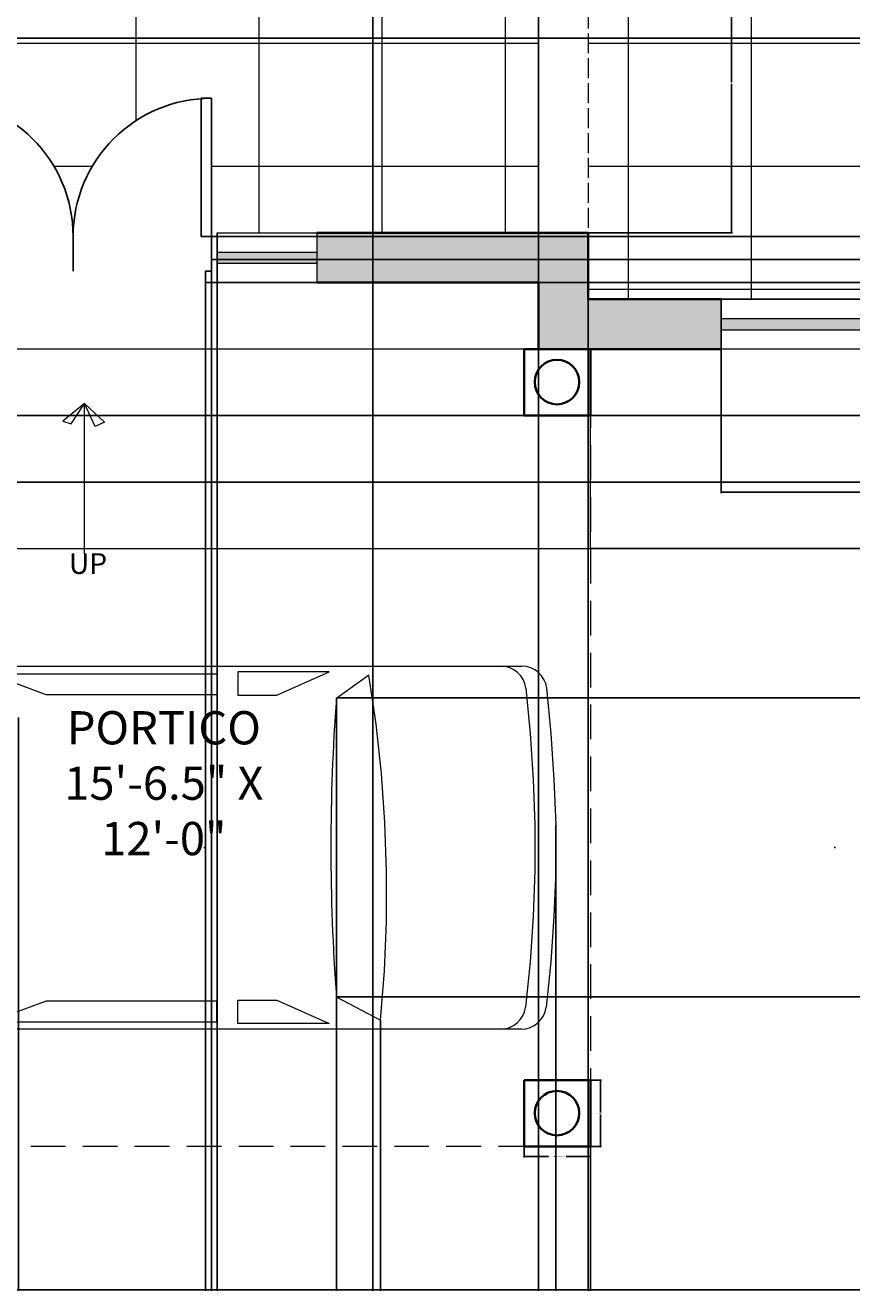
# Model space of a CAD drawing. Units: inches. Extents: x 6 to 575, y 34 to 566.
# Tile 13 of 21: x 282 to 431, y 34 to 262. Entities that reach past the tile are written whole.
import ezdxf

# ---------------------------------------------------------------- set-up
doc = ezdxf.new("R2010")
doc.units = ezdxf.units.IN
doc.linetypes.add('ACAD_ISO02W100', pattern=[15, 12, -3])
for name, color, linetype, lineweight in [('A-ANNO-DIMS', 2, 'Continuous', 18), ('A-ANNO-SYMB', 6, 'Continuous', 18), ('A-ANNO-TEXT', 6, 'Continuous', 18), ('A-AREA-IDEN', 6, 'Continuous', 20), ('A-COLS', 7, 'Continuous', 35), ('A-FLOR-PATT', 252, 'Continuous', 9), ('A-GLAZ-PATT', 4, 'Continuous', 9), ('A-ROOF-OVHD', 240, 'ACAD_ISO02W100', 13), ('A-WALL-OVHD', 7, 'ACAD_ISO02W100', 18), ('A-WALL-PATT', 251, 'Continuous', 9), ('CARS', 5, 'Continuous', 18), ('DOORS', 3, 'Continuous', 25), ('STAIRS', 1, 'Continuous', 20), ('WALLS', 7, 'Continuous', 35), ('WINDOWS', 4, 'Continuous', 20)]:
    doc.layers.add(name, color=color, linetype=linetype, lineweight=lineweight)
doc.styles.add('PDF Arial Narrow', font='txt')
doc.styles.add('PDF Century Gothic', font='txt')
doc.styles.get("Standard").update_dxf_attribs({"font": 'arial.ttf'})
doc.dimstyles.get("Standard").update_dxf_attribs({"dimtxt": 0.18, "dimasz": 0.18, "dimexe": 0.18, "dimexo": 0.0625, "dimgap": 0.09, "dimtad": 0, "dimtih": 1, "dimtoh": 1, "dimdec": 4, "dimzin": 0, "dimdsep": 46, "dimtxsty": 'Standard', "dimcen": 0.09, "dimadec": 0, "dimazin": 0, "dimtfac": 1, "dimtdec": 4, "dimtofl": 0, "dimtmove": 0, "dimatfit": 3, "dimfxl": 1, "dimtolj": 1, "dimtzin": 0, "dimarcsym": 0})
pattern_1 = [(0, (-98.035, 170.147), (0, 22.225), []), (90, (-98.035, 170.147), (-22.225, 1e-15), [])]

# ---------------------------------------------------------------- blocks, each defined once
blk = doc.blocks.new('*U4')
for p, q in [((0, 0), (0, -6)), ((24, 0), (24, -6))]:
    blk.add_line(p, q)
blk.add_lwpolyline([(0, 0), (0, 24), (1.75, 24), (1.75, 0)], close=True)
blk.add_arc((0, 0), 24, 0, 90)
blk = doc.blocks.new('WIN-SIDELIGHT-18IN')
for p, q in [((0, 9), (0, 0)), ((0, 0), (0, 9)), ((0, 9), (0, 0)), ((18, 9), (18, 0)), ((0, 5.5), (18, 5.5)), ((0, 3.5), (18, 3.5))]:
    blk.add_line(p, q)
blk.add_lwpolyline([(0, 9), (18, 9), (18, 0), (0, 0)], close=True)
blk = doc.blocks.new('COL-PORTICO-SQUARE-BASE')
blk.add_lwpolyline([(0, 12.01), (12.02, 12.01), (12.02, 0), (0, 0)], close=True)
blk.add_circle((5.95, 6.05), 4.02)
blk = doc.blocks.new('*D25')
at = {"layer": 'A-ANNO-DIMS', "color": 0, "lineweight": -2, "transparency": 16777216}
for p, q in [((372.06, 59.71), (372.06, 57.79)), ((384.08, 59.71), (384.08, 57.79)), ((372.24, 57.97), (376.47, 57.97)), ((383.9, 57.97), (379.67, 57.97))]:
    blk.add_line(p, q, dxfattribs=at)
at = {"layer": 'A-ANNO-DIMS', "color": 0, "transparency": 16777216}
for points in [[(372.24, 58), (372.24, 57.94), (372.06, 57.97)], [(383.9, 58), (383.9, 57.94), (384.08, 57.97)]]:
    blk.add_solid(points, dxfattribs=at)
at = {"layer": 'Defpoints', "color": 0, "transparency": 16777216}
for p in [(372.06, 59.77), (384.08, 59.78), (384.08, 57.97)]:
    blk.add_point(p, dxfattribs=at)
at = {"layer": 'A-ANNO-DIMS', "color": 0, "transparency": 16777216, "insert": (378.07, 57.97), "char_height": 0.18, "attachment_point": 5}
blk.add_mtext('\\A1;COLUMN BASE R 12 TYP.', dxfattribs=at)
blk = doc.blocks.new('*D26')
at = {"layer": 'A-ANNO-DIMS', "color": 0, "lineweight": -2, "transparency": 16777216}
for p, q in [((384.14, 71.79), (386.06, 71.79)), ((385.88, 71.61), (385.88, 65.96)), ((385.88, 59.96), (385.88, 65.6)), ((384.14, 59.78), (386.06, 59.78))]:
    blk.add_line(p, q, dxfattribs=at)
at = {"layer": 'A-ANNO-DIMS', "color": 0, "transparency": 16777216}
for points in [[(385.91, 71.61), (385.85, 71.61), (385.88, 71.79)], [(385.91, 59.96), (385.85, 59.96), (385.88, 59.78)]]:
    blk.add_solid(points, dxfattribs=at)
at = {"layer": 'Defpoints', "color": 0, "transparency": 16777216}
for p in [(384.07, 71.79), (385.88, 71.79), (384.08, 59.78)]:
    blk.add_point(p, dxfattribs=at)
at = {"layer": 'A-ANNO-DIMS', "color": 0, "transparency": 16777216, "insert": (385.88, 65.78), "char_height": 0.18, "attachment_point": 5}
blk.add_mtext('\\A1;12 TYP.', dxfattribs=at)
blk = doc.blocks.new('*D29')
at = {"layer": 'A-ANNO-DIMS', "color": 0, "lineweight": -2, "transparency": 16777216}
for p, q in [((32.66, 203.74), (32.66, 33.76)), ((548.66, 203.74), (548.66, 33.76)), ((32.84, 33.94), (290.37, 33.94)), ((548.48, 33.94), (290.95, 33.94))]:
    blk.add_line(p, q, dxfattribs=at)
at = {"layer": 'A-ANNO-DIMS', "color": 0, "transparency": 16777216}
for points in [[(32.84, 33.97), (32.84, 33.91), (32.66, 33.94)], [(548.48, 33.97), (548.48, 33.91), (548.66, 33.94)]]:
    blk.add_solid(points, dxfattribs=at)
at = {"layer": 'Defpoints', "color": 0, "transparency": 16777216}
for p in [(32.66, 203.8), (548.66, 203.8), (548.66, 33.94)]:
    blk.add_point(p, dxfattribs=at)
at = {"layer": 'A-ANNO-DIMS', "color": 0, "transparency": 16777216, "insert": (290.66, 33.94), "char_height": 0.18, "attachment_point": 5}
blk.add_mtext('\\A1;516', dxfattribs=at)
blk = doc.blocks.new('*D40')
at = {"layer": 'A-ANNO-DIMS', "color": 0, "lineweight": -2, "transparency": 16777216}
for p, q in [((407.66, 203.74), (407.66, 177.79)), ((515.66, 203.74), (515.66, 177.79)), ((407.84, 177.97), (461.38, 177.97)), ((515.48, 177.97), (461.94, 177.97))]:
    blk.add_line(p, q, dxfattribs=at)
at = {"layer": 'A-ANNO-DIMS', "color": 0, "transparency": 16777216}
for points in [[(407.84, 178), (407.84, 177.94), (407.66, 177.97)], [(515.48, 178), (515.48, 177.94), (515.66, 177.97)]]:
    blk.add_solid(points, dxfattribs=at)
at = {"layer": 'Defpoints', "color": 0, "transparency": 16777216}
for p in [(407.66, 203.8), (515.66, 203.8), (407.66, 177.97)]:
    blk.add_point(p, dxfattribs=at)
at = {"layer": 'A-ANNO-DIMS', "color": 0, "transparency": 16777216, "insert": (461.66, 177.97), "char_height": 0.18, "attachment_point": 5}
blk.add_mtext('\\A1;108', dxfattribs=at)
blk = doc.blocks.new('*D48')
at = {"layer": 'A-ANNO-DIMS', "color": 0, "lineweight": -2, "transparency": 16777216}
for p, q in [((264.66, 215.74), (264.66, 33.76)), ((316.66, 215.74), (316.66, 33.76)), ((264.84, 33.94), (290.44, 33.94)), ((316.48, 33.94), (290.88, 33.94))]:
    blk.add_line(p, q, dxfattribs=at)
at = {"layer": 'A-ANNO-DIMS', "color": 0, "transparency": 16777216}
for points in [[(264.84, 33.97), (264.84, 33.91), (264.66, 33.94)], [(316.48, 33.97), (316.48, 33.91), (316.66, 33.94)]]:
    blk.add_solid(points, dxfattribs=at)
at = {"layer": 'Defpoints', "color": 0, "transparency": 16777216}
for p in [(264.66, 215.8), (316.66, 215.8), (316.66, 33.94)]:
    blk.add_point(p, dxfattribs=at)
at = {"layer": 'A-ANNO-DIMS', "color": 0, "transparency": 16777216, "insert": (290.66, 33.94), "char_height": 0.18, "attachment_point": 5}
blk.add_mtext('\\A1;52', dxfattribs=at)
blk = doc.blocks.new('*D54')
at = {"layer": 'A-ANNO-DIMS', "color": 0, "lineweight": -2, "transparency": 16777216}
for p, q in [((444.96, 337.94), (6.65, 337.94)), ((6.83, 337.76), (6.83, 299.11)), ((6.83, 260.1), (6.83, 298.75)), ((444.96, 259.92), (6.65, 259.92))]:
    blk.add_line(p, q, dxfattribs=at)
at = {"layer": 'A-ANNO-DIMS', "color": 0, "transparency": 16777216}
for points in [[(6.8, 337.76), (6.86, 337.76), (6.83, 337.94)], [(6.8, 260.1), (6.86, 260.1), (6.83, 259.92)]]:
    blk.add_solid(points, dxfattribs=at)
at = {"layer": 'Defpoints', "color": 0, "transparency": 16777216}
for p in [(6.83, 337.94), (445.02, 337.94), (445.02, 259.92)]:
    blk.add_point(p, dxfattribs=at)
at = {"layer": 'A-ANNO-DIMS', "color": 0, "transparency": 16777216, "insert": (6.83, 298.93), "char_height": 0.18, "attachment_point": 5}
blk.add_mtext('\\A1;78.02', dxfattribs=at)
blk = doc.blocks.new('*D58')
at = {"layer": 'A-ANNO-DIMS', "color": 0, "lineweight": -2, "transparency": 16777216}
for p, q in [((383.72, 278.8), (409.67, 278.8)), ((409.49, 278.62), (409.49, 251.98)), ((409.49, 224.98), (409.49, 251.62)), ((383.72, 224.8), (409.67, 224.8))]:
    blk.add_line(p, q, dxfattribs=at)
at = {"layer": 'A-ANNO-DIMS', "color": 0, "transparency": 16777216}
for points in [[(409.46, 278.62), (409.52, 278.62), (409.49, 278.8)], [(409.46, 224.98), (409.52, 224.98), (409.49, 224.8)]]:
    blk.add_solid(points, dxfattribs=at)
at = {"layer": 'Defpoints', "color": 0, "transparency": 16777216}
for p in [(383.66, 278.8), (383.66, 224.8), (409.49, 224.8)]:
    blk.add_point(p, dxfattribs=at)
at = {"layer": 'A-ANNO-DIMS', "color": 0, "transparency": 16777216, "insert": (409.49, 251.8), "char_height": 0.18, "attachment_point": 5}
blk.add_mtext('\\A1;54', dxfattribs=at)
blk = doc.blocks.new('*D74')
at = {"layer": 'A-ANNO-DIMS', "color": 0, "lineweight": -2, "transparency": 16777216}
for p, q in [((384.14, 191.79), (574.68, 191.79)), ((574.5, 191.61), (574.5, 185.96)), ((574.5, 179.95), (574.5, 185.6)), ((384.14, 179.77), (574.68, 179.77))]:
    blk.add_line(p, q, dxfattribs=at)
at = {"layer": 'A-ANNO-DIMS', "color": 0, "transparency": 16777216}
for points in [[(574.47, 191.61), (574.53, 191.61), (574.5, 191.79)], [(574.47, 179.95), (574.53, 179.95), (574.5, 179.77)]]:
    blk.add_solid(points, dxfattribs=at)
at = {"layer": 'Defpoints', "color": 0, "transparency": 16777216}
for p in [(384.08, 191.79), (384.08, 179.77), (574.5, 179.77)]:
    blk.add_point(p, dxfattribs=at)
at = {"layer": 'A-ANNO-DIMS', "color": 0, "transparency": 16777216, "insert": (574.5, 185.78), "char_height": 0.18, "attachment_point": 5}
blk.add_mtext('\\A1;12.015', dxfattribs=at)
blk = doc.blocks.new('*D75')
at = {"layer": 'A-ANNO-DIMS', "color": 0, "lineweight": -2, "transparency": 16777216}
for p, q in [((384.14, 179.77), (574.68, 179.77)), ((574.5, 179.59), (574.5, 173.95)), ((574.5, 167.94), (574.5, 173.58)), ((384.14, 167.76), (574.68, 167.76))]:
    blk.add_line(p, q, dxfattribs=at)
at = {"layer": 'A-ANNO-DIMS', "color": 0, "transparency": 16777216}
for points in [[(574.47, 179.59), (574.53, 179.59), (574.5, 179.77)], [(574.47, 167.94), (574.53, 167.94), (574.5, 167.76)]]:
    blk.add_solid(points, dxfattribs=at)
at = {"layer": 'Defpoints', "color": 0, "transparency": 16777216}
for p in [(384.08, 179.77), (384.08, 167.76), (574.5, 167.76)]:
    blk.add_point(p, dxfattribs=at)
at = {"layer": 'A-ANNO-DIMS', "color": 0, "transparency": 16777216, "insert": (574.5, 173.76), "char_height": 0.18, "attachment_point": 5}
blk.add_mtext('\\A1;12.015', dxfattribs=at)
blk = doc.blocks.new('*D76')
at = {"layer": 'A-ANNO-DIMS', "color": 0, "lineweight": -2, "transparency": 16777216}
for p, q in [((197.69, 59.71), (197.69, 33.76)), ((384.08, 59.71), (384.08, 33.76)), ((197.87, 33.94), (290.5, 33.94)), ((383.9, 33.94), (291.27, 33.94))]:
    blk.add_line(p, q, dxfattribs=at)
at = {"layer": 'A-ANNO-DIMS', "color": 0, "transparency": 16777216}
for points in [[(197.87, 33.97), (197.87, 33.91), (197.69, 33.94)], [(383.9, 33.97), (383.9, 33.91), (384.08, 33.94)]]:
    blk.add_solid(points, dxfattribs=at)
at = {"layer": 'Defpoints', "color": 0, "transparency": 16777216}
for p in [(197.69, 59.77), (384.08, 59.78), (384.08, 33.94)]:
    blk.add_point(p, dxfattribs=at)
at = {"layer": 'A-ANNO-DIMS', "color": 0, "transparency": 16777216, "insert": (290.88, 33.94), "char_height": 0.18, "attachment_point": 5}
blk.add_mtext('\\A1;186.4', dxfattribs=at)
blk = doc.blocks.new('*D78')
at = {"layer": 'A-ANNO-DIMS', "color": 0, "lineweight": -2, "transparency": 16777216}
for p, q in [((377.83, 117.84), (377.83, 33.76)), ((206.58, 113.74), (206.58, 33.76)), ((206.76, 33.94), (291.75, 33.94)), ((377.65, 33.94), (292.66, 33.94))]:
    blk.add_line(p, q, dxfattribs=at)
at = {"layer": 'A-ANNO-DIMS', "color": 0, "transparency": 16777216}
for points in [[(206.76, 33.97), (206.76, 33.91), (206.58, 33.94)], [(377.65, 33.97), (377.65, 33.91), (377.83, 33.94)]]:
    blk.add_solid(points, dxfattribs=at)
at = {"layer": 'Defpoints', "color": 0, "transparency": 16777216}
for p in [(377.83, 117.9), (206.58, 113.81), (377.83, 33.94)]:
    blk.add_point(p, dxfattribs=at)
at = {"layer": 'A-ANNO-DIMS', "color": 0, "transparency": 16777216, "insert": (292.21, 33.94), "char_height": 0.18, "attachment_point": 5}
blk.add_mtext('\\A1;171.25', dxfattribs=at)
blk = doc.blocks.new('*D82')
at = {"layer": 'A-ANNO-DIMS', "color": 0, "lineweight": -2, "transparency": 16777216}
for p, q in [((338.25, 140.81), (574.68, 140.81)), ((574.5, 140.63), (574.5, 113.99)), ((574.5, 86.98), (574.5, 113.62)), ((338.25, 86.8), (574.68, 86.8))]:
    blk.add_line(p, q, dxfattribs=at)
at = {"layer": 'A-ANNO-DIMS', "color": 0, "transparency": 16777216}
for points in [[(574.47, 140.63), (574.53, 140.63), (574.5, 140.81)], [(574.47, 86.98), (574.53, 86.98), (574.5, 86.8)]]:
    blk.add_solid(points, dxfattribs=at)
at = {"layer": 'Defpoints', "color": 0, "transparency": 16777216}
for p in [(338.19, 140.81), (574.5, 140.81), (338.19, 86.8)]:
    blk.add_point(p, dxfattribs=at)
at = {"layer": 'A-ANNO-DIMS', "color": 0, "transparency": 16777216, "insert": (574.5, 113.81), "char_height": 0.18, "attachment_point": 5}
blk.add_mtext('\\A1;54.02', dxfattribs=at)
blk = doc.blocks.new('*D85')
at = {"layer": 'A-ANNO-DIMS', "color": 0, "lineweight": -2, "transparency": 16777216}
for p, q in [((338.19, 140.75), (338.19, 33.76)), ((280.78, 137.27), (280.78, 33.76)), ((280.96, 33.94), (309.11, 33.94)), ((338.01, 33.94), (309.86, 33.94))]:
    blk.add_line(p, q, dxfattribs=at)
at = {"layer": 'A-ANNO-DIMS', "color": 0, "transparency": 16777216}
for points in [[(280.96, 33.97), (280.96, 33.91), (280.78, 33.94)], [(338.01, 33.97), (338.01, 33.91), (338.19, 33.94)]]:
    blk.add_solid(points, dxfattribs=at)
at = {"layer": 'Defpoints', "color": 0, "transparency": 16777216}
for p in [(338.19, 140.81), (280.78, 137.33), (338.19, 33.94)]:
    blk.add_point(p, dxfattribs=at)
at = {"layer": 'A-ANNO-DIMS', "color": 0, "transparency": 16777216, "insert": (309.48, 33.94), "char_height": 0.18, "attachment_point": 5}
blk.add_mtext('\\A1;57.41', dxfattribs=at)
blk = doc.blocks.new('*D86')
at = {"layer": 'A-ANNO-DIMS', "color": 0, "lineweight": -2, "transparency": 16777216}
for p, q in [((338.19, 86.73), (338.19, 33.76)), ((346.16, 82.57), (346.16, 33.76)), ((338.37, 33.94), (341.78, 33.94)), ((345.98, 33.94), (342.57, 33.94))]:
    blk.add_line(p, q, dxfattribs=at)
at = {"layer": 'A-ANNO-DIMS', "color": 0, "transparency": 16777216}
for points in [[(338.37, 33.97), (338.37, 33.91), (338.19, 33.94)], [(345.98, 33.97), (345.98, 33.91), (346.16, 33.94)]]:
    blk.add_solid(points, dxfattribs=at)
at = {"layer": 'Defpoints', "color": 0, "transparency": 16777216}
for p in [(338.19, 86.8), (346.16, 82.64), (346.16, 33.94)]:
    blk.add_point(p, dxfattribs=at)
at = {"layer": 'A-ANNO-DIMS', "color": 0, "transparency": 16777216, "insert": (342.17, 33.94), "char_height": 0.18, "attachment_point": 5}
blk.add_mtext('\\A1;7.967', dxfattribs=at)
blk = doc.blocks.new('*D122')
at = {"layer": 'A-ANNO-DIMS', "color": 0, "lineweight": -2, "transparency": 16777216}
for p, q in [((344.78, 281.17), (344.78, 33.76)), ((374.66, 278.74), (374.66, 33.76)), ((344.96, 33.94), (359.32, 33.94)), ((374.48, 33.94), (360.11, 33.94))]:
    blk.add_line(p, q, dxfattribs=at)
at = {"layer": 'A-ANNO-DIMS', "color": 0, "transparency": 16777216}
for points in [[(344.96, 33.97), (344.96, 33.91), (344.78, 33.94)], [(374.48, 33.97), (374.48, 33.91), (374.66, 33.94)]]:
    blk.add_solid(points, dxfattribs=at)
at = {"layer": 'Defpoints', "color": 0, "transparency": 16777216}
for p in [(344.78, 281.24), (374.66, 278.8), (344.78, 33.94)]:
    blk.add_point(p, dxfattribs=at)
at = {"layer": 'A-ANNO-DIMS', "color": 0, "transparency": 16777216, "insert": (359.72, 33.94), "char_height": 0.18, "attachment_point": 5}
blk.add_mtext('\\A1;29.88', dxfattribs=at)
blk = doc.blocks.new('*D138')
at = {"layer": 'A-ANNO-DIMS', "color": 0, "lineweight": -2, "transparency": 16777216}
for p, q in [((445.02, 259.86), (445.02, 33.76)), ((383.66, 212.74), (383.66, 33.76)), ((383.84, 33.94), (413.95, 33.94)), ((444.84, 33.94), (414.73, 33.94))]:
    blk.add_line(p, q, dxfattribs=at)
at = {"layer": 'A-ANNO-DIMS', "color": 0, "transparency": 16777216}
for points in [[(383.84, 33.97), (383.84, 33.91), (383.66, 33.94)], [(444.84, 33.97), (444.84, 33.91), (445.02, 33.94)]]:
    blk.add_solid(points, dxfattribs=at)
at = {"layer": 'Defpoints', "color": 0, "transparency": 16777216}
for p in [(445.02, 259.92), (383.66, 212.8), (445.02, 33.94)]:
    blk.add_point(p, dxfattribs=at)
at = {"layer": 'A-ANNO-DIMS', "color": 0, "transparency": 16777216, "insert": (414.34, 33.94), "char_height": 0.18, "attachment_point": 5}
blk.add_mtext('\\A1;61.36', dxfattribs=at)
blk = doc.blocks.new('*D139')
at = {"layer": 'A-ANNO-DIMS', "color": 0, "lineweight": -2, "transparency": 16777216}
for p, q in [((445.08, 259.92), (574.68, 259.92)), ((574.5, 259.74), (574.5, 236.54)), ((574.5, 212.98), (574.5, 236.18)), ((383.72, 212.8), (574.68, 212.8))]:
    blk.add_line(p, q, dxfattribs=at)
at = {"layer": 'A-ANNO-DIMS', "color": 0, "transparency": 16777216}
for points in [[(574.47, 259.74), (574.53, 259.74), (574.5, 259.92)], [(574.47, 212.98), (574.53, 212.98), (574.5, 212.8)]]:
    blk.add_solid(points, dxfattribs=at)
at = {"layer": 'Defpoints', "color": 0, "transparency": 16777216}
for p in [(445.02, 259.92), (574.5, 259.92), (383.66, 212.8)]:
    blk.add_point(p, dxfattribs=at)
at = {"layer": 'A-ANNO-DIMS', "color": 0, "transparency": 16777216, "insert": (574.5, 236.36), "char_height": 0.18, "attachment_point": 5}
blk.add_mtext('\\A1;47.12', dxfattribs=at)
blk = doc.blocks.new('*D211')
at = {"layer": 'A-ANNO-DIMS', "color": 0, "lineweight": -2, "transparency": 16777216}
for p, q in [((314.58, 215.74), (314.58, 33.76)), ((316.66, 215.74), (316.66, 33.76)), ((314.76, 33.94), (315.29, 33.94)), ((316.48, 33.94), (315.94, 33.94))]:
    blk.add_line(p, q, dxfattribs=at)
at = {"layer": 'A-ANNO-DIMS', "color": 0, "transparency": 16777216}
for points in [[(314.76, 33.97), (314.76, 33.91), (314.58, 33.94)], [(316.48, 33.97), (316.48, 33.91), (316.66, 33.94)]]:
    blk.add_solid(points, dxfattribs=at)
at = {"layer": 'Defpoints', "color": 0, "transparency": 16777216}
for p in [(314.58, 215.8), (316.66, 215.8), (314.58, 33.94)]:
    blk.add_point(p, dxfattribs=at)
at = {"layer": 'A-ANNO-DIMS', "color": 0, "transparency": 16777216, "insert": (315.62, 33.94), "char_height": 0.18, "attachment_point": 5}
blk.add_mtext('\\A1;2.08', dxfattribs=at)
blk = doc.blocks.new('*D212')
at = {"layer": 'A-ANNO-DIMS', "color": 0, "lineweight": -2, "transparency": 16777216}
for p, q in [((316.72, 219.96), (574.68, 219.96)), ((574.5, 219.78), (574.5, 218.06)), ((574.5, 215.98), (574.5, 217.7)), ((316.72, 215.8), (574.68, 215.8))]:
    blk.add_line(p, q, dxfattribs=at)
at = {"layer": 'A-ANNO-DIMS', "color": 0, "transparency": 16777216}
for points in [[(574.47, 219.78), (574.53, 219.78), (574.5, 219.96)], [(574.47, 215.98), (574.53, 215.98), (574.5, 215.8)]]:
    blk.add_solid(points, dxfattribs=at)
at = {"layer": 'Defpoints', "color": 0, "transparency": 16777216}
for p in [(316.66, 219.96), (574.5, 219.96), (316.66, 215.8)]:
    blk.add_point(p, dxfattribs=at)
at = {"layer": 'A-ANNO-DIMS', "color": 0, "transparency": 16777216, "insert": (574.5, 217.88), "char_height": 0.18, "attachment_point": 5}
blk.add_mtext('\\A1;4.16', dxfattribs=at)
blk = doc.blocks.new('*D213')
at = {"layer": 'A-ANNO-DIMS', "color": 0, "lineweight": -2, "transparency": 16777216}
for p, q in [((314.578645, 217.818484), (314.578645, 33.76465)), ((315.618645, 217.818484), (315.618645, 33.76465)), ((314.398645, 33.94465), (314.218645, 33.94465)), ((315.798645, 33.94465), (315.978645, 33.94465))]:
    blk.add_line(p, q, dxfattribs=at)
at = {"layer": 'A-ANNO-DIMS', "color": 0, "transparency": 16777216}
for points in [[(314.398645, 33.97465), (314.398645, 33.91465), (314.578645, 33.94465)], [(315.798645, 33.97465), (315.798645, 33.91465), (315.618645, 33.94465)]]:
    blk.add_solid(points, dxfattribs=at)
at = {"layer": 'Defpoints', "color": 0, "transparency": 16777216}
for p in [(314.578645, 217.880984), (315.618645, 217.880984), (314.578645, 33.94465)]:
    blk.add_point(p, dxfattribs=at)
at = {"layer": 'A-ANNO-DIMS', "color": 0, "transparency": 16777216, "insert": (315.098645, 33.94465), "char_height": 0.18, "attachment_point": 5}
blk.add_mtext('\\A1;1.04', dxfattribs=at)
blk = doc.blocks.new('*D216')
at = {"layer": 'A-ANNO-DIMS', "color": 0, "lineweight": -2, "transparency": 16777216}
for p, q in [((315.68, 224.12), (574.68, 224.12)), ((574.5, 223.94), (574.5, 222.22)), ((574.5, 220.14), (574.5, 221.86)), ((315.68, 219.96), (574.68, 219.96))]:
    blk.add_line(p, q, dxfattribs=at)
at = {"layer": 'A-ANNO-DIMS', "color": 0, "transparency": 16777216}
for points in [[(574.47, 223.94), (574.53, 223.94), (574.5, 224.12)], [(574.47, 220.14), (574.53, 220.14), (574.5, 219.96)]]:
    blk.add_solid(points, dxfattribs=at)
at = {"layer": 'Defpoints', "color": 0, "transparency": 16777216}
for p in [(315.62, 224.12), (574.5, 224.12), (315.62, 219.96)]:
    blk.add_point(p, dxfattribs=at)
at = {"layer": 'A-ANNO-DIMS', "color": 0, "transparency": 16777216, "insert": (574.5, 222.04), "char_height": 0.18, "attachment_point": 5}
blk.add_mtext('\\A1;4.16', dxfattribs=at)
blk = doc.blocks.new('*D220')
at = {"layer": 'A-ANNO-DIMS', "color": 0, "lineweight": -2, "transparency": 16777216}
for p, q in [((155, 113.8), (257.27, 113.8)), ((428.11, 113.81), (428.29, 113.81)), ((428.2, 113.72), (428.2, 113.9))]:
    blk.add_line(p, q, dxfattribs=at)
at = {"layer": 'A-ANNO-DIMS', "color": 0, "transparency": 16777216}
blk.add_solid([(257.27, 113.83), (257.27, 113.77), (257.45, 113.8)], dxfattribs=at)
at = {"layer": 'Defpoints', "color": 0, "transparency": 16777216}
for p in [(257.45, 113.8), (428.2, 113.81)]:
    blk.add_point(p, dxfattribs=at)
at = {"layer": 'A-ANNO-DIMS', "color": 0, "transparency": 16777216, "insert": (154.45, 113.8), "char_height": 0.18, "attachment_point": 5}
blk.add_mtext('\\A1;R170.75', dxfattribs=at)
blk = doc.blocks.new('*D221')
at = {"layer": 'A-ANNO-DIMS', "color": 0, "lineweight": -2, "transparency": 16777216}
for p, q in [((141.91, 113.8), (206.4, 113.8)), ((314.28, 113.81), (314.46, 113.81)), ((314.37, 113.72), (314.37, 113.9))]:
    blk.add_line(p, q, dxfattribs=at)
at = {"layer": 'A-ANNO-DIMS', "color": 0, "transparency": 16777216}
blk.add_solid([(206.4, 113.83), (206.4, 113.77), (206.58, 113.8)], dxfattribs=at)
at = {"layer": 'Defpoints', "color": 0, "transparency": 16777216}
for p in [(206.58, 113.8), (314.37, 113.81)]:
    blk.add_point(p, dxfattribs=at)
at = {"layer": 'A-ANNO-DIMS', "color": 0, "transparency": 16777216, "insert": (141.36, 113.8), "char_height": 0.18, "attachment_point": 5}
blk.add_mtext('\\A1;R107.78', dxfattribs=at)
blk = doc.blocks.new('*D222')
at = {"layer": 'A-ANNO-DIMS', "color": 0, "lineweight": -2, "transparency": 16777216}
for p, q in [((150.38, 113.8), (211.32, 113.8)), ((313.26, 113.81), (313.44, 113.81)), ((313.35, 113.72), (313.35, 113.9))]:
    blk.add_line(p, q, dxfattribs=at)
at = {"layer": 'A-ANNO-DIMS', "color": 0, "transparency": 16777216}
blk.add_solid([(211.32, 113.83), (211.32, 113.77), (211.5, 113.8)], dxfattribs=at)
at = {"layer": 'Defpoints', "color": 0, "transparency": 16777216}
for p in [(211.5, 113.8), (313.35, 113.81)]:
    blk.add_point(p, dxfattribs=at)
at = {"layer": 'A-ANNO-DIMS', "color": 0, "transparency": 16777216, "insert": (149.83, 113.8), "char_height": 0.18, "attachment_point": 5}
blk.add_mtext('\\A1;R101.85', dxfattribs=at)

msp = doc.modelspace()

# ---------------------------------------------------------------- hatches: boundary and pattern name
at = {"layer": 'A-FLOR-PATT'}
h = msp.add_hatch(dxfattribs=at)
h.set_pattern_fill('NET', color=256, scale=7)
h.set_pattern_definition(pattern_1)
h.paths.add_polyline_path([(539.6586, 366.801), (539.6586, 378.801), (433.708, 378.801), (383.6586, 378.801), (383.6586, 278.801), (383.6586, 224.801), (383.6586, 212.801), (407.6586, 212.801), (515.6586, 212.801), (539.6586, 212.801), (539.6586, 270.801)])
h.paths.add_polyline_path([(434.8003, 333.3365), (436.6727, 333.3365), (436.6727, 331.9322), (445.0208, 331.9322), (445.0208, 337.9397), (456.1776, 337.9397), (456.1776, 346.2878), (454.7733, 346.2878), (454.7733, 348.1603), (474.2782, 348.1603), (474.2782, 346.2878), (472.8738, 346.2878), (472.8738, 337.9397), (484.0307, 337.9397), (484.0307, 331.9322), (492.3788, 331.9322), (492.3788, 333.3365), (494.2512, 333.3365), (494.2512, 313.8316), (492.3788, 313.8316), (492.3788, 315.158), (484.0307, 315.158), (484.0307, 307.278), (492.3788, 307.278), (492.3788, 308.6823), (494.2512, 308.6823), (494.2512, 289.1774), (492.3788, 289.1774), (492.3788, 290.5818), (484.0307, 290.5818), (484.0307, 282.7018), (492.3788, 282.7018), (492.3788, 284.1062), (494.2512, 284.1062), (494.2512, 264.6013), (492.3788, 264.6013), (492.3788, 266.0056), (484.0307, 266.0056), (484.0307, 259.9201), (472.8738, 259.9201), (472.8738, 251.572), (474.2782, 251.572), (474.2782, 249.6995), (454.7733, 249.6995), (454.7733, 251.572), (456.1776, 251.572), (456.1776, 259.9201), (445.0208, 259.9201), (445.0208, 266.0056), (436.6727, 266.0056), (436.6727, 264.6013), (434.8003, 264.6013), (434.8003, 284.1062), (436.6727, 284.1062), (436.6727, 282.7018), (445.0208, 282.7018), (445.0208, 290.5818), (436.6727, 290.5818), (436.6727, 289.1774), (434.8003, 289.1774), (434.8003, 308.6823), (436.6727, 308.6823), (436.6727, 307.278), (445.0208, 307.278), (445.0208, 315.158), (436.6727, 315.158), (436.6727, 313.8316), (434.8003, 313.8316)], flags=16)
h.paths.add_polyline_path([(532.9619, 436.5144), (533.9192, 437.0672), (533.9307, 437.0472, -0.12106636), (546.2274, 440.0689), (539.6586, 440.801), (539.6586, 450.6781), (515.7066, 450.6781), (515.7066, 507.3203), (407.6494, 507.3203), (407.6494, 449.3517), (383.6586, 449.3517), (383.6586, 382.801), (433.708, 382.801), (433.708, 406.831), (539.6586, 406.831), (539.6586, 412.801), (545.7108, 412.801), (545.7108, 414.4327)])
h.paths.add_polyline_path([(437.687, 435.3082), (437.687, 471.3533), (485.6691, 471.3533), (485.6691, 435.3082)], flags=16)
h = msp.add_hatch(dxfattribs=at)
h.set_pattern_fill('NET', color=256, scale=7)
h.set_pattern_definition(pattern_1)
h.paths.add_polyline_path([(368.183, 395.6385, -0.88370529), (374.2533, 394.8861), (374.6586, 448.801), (354.6586, 448.801), (354.6586, 448.7938), (353.1847, 448.7938), (326.6586, 448.801), (322.6586, 448.801), (248.6332, 448.8024), (206.6586, 448.8024), (206.6586, 389.449), (221.6622, 389.449), (221.6622, 310.5712), (206.6586, 310.5712), (206.6586, 276.801), (206.6704, 276.801), (206.6704, 274.3795), (206.6586, 224.801), (246.6586, 224.801), (264.6586, 224.801), (265.6986, 224.801), (265.6986, 249.081), (267.5186, 249.081), (267.5186, 249.0145, -0.38515288), (290.6494, 224.801), (290.6679, 224.801, -0.38515288), (313.7986, 249.0145), (313.7986, 249.081), (315.6186, 249.081), (315.6186, 224.801), (316.6586, 224.801), (334.6586, 224.801), (374.6586, 224.801), (374.6586, 278.801), (374.1753, 318.8919, -0.45530286), (370.7577, 315.9168), (370.6643, 313.8205, -0.41421356), (368.7528, 311.909), (368.8072, 311.8975), (368.7528, 311.909, 0.41421356), (370.6643, 313.8205), (370.7632, 315.9161, -0.34634601), (368.183, 318.5897)])
h.paths.add_polyline_path([(288.603, 342.0131), (288.603, 389.9952), (318.6406, 389.9952), (318.6406, 342.0131)], flags=16)
h.paths.add_polyline_path([(289.6173, 343.0274), (289.6173, 389.059), (317.6263, 389.059), (317.6263, 343.0274)], flags=0)
h.paths.add_polyline_path([(295.4867, 311.7535, 0.06538163), (295.1241, 312.0945), (295.0006, 312.1316)], flags=16)
h.paths.add_polyline_path([(328.4931, 284.9911, 0.41421356), (330.4045, 286.9026), (330.4215, 286.8532), (330.4045, 286.9026, -0.41421356), (328.4931, 284.9911), (328.549, 284.9808)], flags=16)
h.paths.add_polyline_path([(344.7771, 305.2659), (368.8072, 305.2659), (368.8072, 281.2358), (344.7771, 281.2358)], flags=16)
h.paths.add_polyline_path([(368.183, 288.1406, -1), (356.246, 288.1406, -1)], flags=0)
h.paths.add_polyline_path([(347.9759, 404.6629), (347.9759, 428.6929), (372.006, 428.6929), (372.006, 404.6629)], flags=16)
h.paths.add_polyline_path([(359.4448, 421.7882, -1), (371.3818, 421.7882, -1)], flags=0)
at = {"layer": 'A-GLAZ-PATT'}
h = msp.add_hatch(color=256, dxfattribs=at)
h.dxf.hatch_style = 1
h.paths.add_polyline_path([(36.1586, 224.801), (38.1586, 224.801), (38.1586, 272.801), (36.1586, 272.801)])
h.paths.add_polyline_path([(167.6586, 207.301), (167.6586, 209.301), (71.6586, 209.301), (71.6586, 207.301)])
h.paths.add_polyline_path([(264.6586, 219.301), (264.6586, 221.301), (246.6586, 221.301), (246.6586, 219.301)])
h.paths.add_polyline_path([(316.6586, 221.301), (316.6586, 219.301), (334.6586, 219.301), (334.6586, 221.301)])
h.paths.add_polyline_path([(515.6586, 207.301), (515.6586, 209.301), (407.6586, 209.301), (407.6586, 207.301)])
h.paths.add_polyline_path([(543.1586, 270.801), (545.1586, 270.801), (545.1586, 366.801), (543.1586, 366.801)])
h.paths.add_polyline_path([(407.9436, 536.301), (407.9436, 534.301), (455.9436, 534.301), (455.9436, 536.301)])
h.paths.add_polyline_path([(272.6586, 536.301), (272.6586, 534.301), (320.6586, 534.301), (320.6586, 536.301)])
at = {"layer": 'A-WALL-PATT'}
h = msp.add_hatch(color=256, dxfattribs=at)
h.dxf.hatch_style = 1
h.paths.add_polyline_path([(160.6586, 539.801), (32.6586, 539.801), (32.6586, 272.801), (41.6586, 272.801), (41.6586, 286.0643), (41.6586, 358.0764), (41.6586, 379.0637), (41.6586, 407.7709), (41.6194, 407.7709), (41.6194, 431.801), (82.8918, 431.801), (82.8918, 440.801), (65.6494, 440.801), (65.6494, 440.7732), (41.6194, 440.7732), (41.6194, 515.5941), (41.6586, 530.801), (117.6586, 530.801), (117.6586, 474.801), (120.6068, 474.801), (121.6586, 474.801), (121.6586, 530.801), (137.4275, 530.801), (137.4275, 530.8356), (141.2505, 530.8356), (160.6586, 530.801)])
h.paths.add_polyline_path([(71.6586, 212.801), (41.6586, 212.801), (41.6586, 224.801), (32.6586, 224.801), (32.6586, 203.801), (71.6586, 203.801)])
h.paths.add_polyline_path([(206.6586, 215.801), (246.6586, 215.801), (246.6586, 224.801), (206.6586, 224.801), (206.6586, 230.801), (201.8157, 230.801), (197.6586, 230.801), (197.6586, 212.801), (167.6586, 212.801), (167.6586, 203.801), (206.6586, 203.801)])
h.paths.add_polyline_path([(383.6586, 224.801), (334.6586, 224.801), (334.6586, 215.801), (374.6586, 215.801), (374.6586, 203.801), (384.0753, 203.801), (407.6586, 203.801), (407.6586, 212.801), (383.6586, 212.801)])
h.paths.add_polyline_path([(548.6586, 270.801), (539.6586, 270.801), (539.6586, 212.801), (515.6586, 212.801), (515.6586, 203.801), (548.6586, 203.801)])
h.paths.add_polyline_path([(548.6586, 412.801), (545.7108, 412.801), (539.6586, 412.801), (539.6586, 382.801), (433.708, 382.801), (433.708, 378.801), (539.6586, 378.801), (539.6586, 366.801), (548.6586, 366.801)])
h.paths.add_polyline_path([(548.6586, 539.801), (455.9436, 539.801), (455.9436, 530.801), (539.6586, 530.801), (539.6586, 440.801), (548.6586, 440.801)])
h.paths.add_polyline_path([(407.9436, 539.801), (362.6586, 539.801), (362.6586, 530.801), (374.6586, 530.801), (374.6586, 452.801), (354.6586, 452.801), (354.6586, 448.801), (374.6586, 448.801), (374.6586, 278.801), (383.6586, 278.801), (383.6586, 530.801), (407.9436, 530.801)])
h.paths.add_polyline_path([(338.6586, 539.801), (320.6586, 539.801), (320.6586, 530.801), (322.6586, 530.801), (322.6586, 448.801), (326.6586, 448.801), (326.6586, 530.801), (338.6586, 530.801)])
h.paths.add_polyline_path([(272.6586, 539.801), (184.6586, 539.801), (184.6586, 530.801), (197.6586, 530.801), (197.6586, 440.801), (176.6714, 440.801), (121.6586, 440.801), (121.6586, 446.801), (117.6586, 446.801), (117.6586, 440.801), (111.6586, 440.801), (111.6586, 431.801), (197.6586, 431.801), (197.6586, 407.7709), (197.6586, 276.801), (206.6586, 276.801), (206.6586, 530.801), (272.6586, 530.801)])

# ---------------------------------------------------------------- linework, layer by layer
at = {"layer": 'A-ANNO-SYMB'}
msp.add_lwpolyline([(292.7143, 166.8977), (292.7143, 193.9705), (288.8133, 190.7717), (290.2957, 190.3036), (292.7143, 193.9705), (296.3032, 190.6157), (294.6648, 189.8355), (292.7143, 193.9705)], dxfattribs=at)
at = {"layer": 'A-ROOF-OVHD'}
for points in [[(384.0753, 195.843), (384.0753, 189.6014)], [(384.0753, 186.4806), (384.0753, 180.2391)], [(384.0753, 177.0403), (384.0753, 170.7987)], [(384.0753, 167.6779), (384.0753, 161.4363)], [(384.0753, 158.3155), (384.0753, 152.074)], [(384.0753, 148.9532), (384.0753, 142.7116)], [(384.0753, 139.5908), (384.0753, 133.3493)], [(384.0753, 130.2285), (384.0753, 123.9869)], [(384.0753, 120.8661), (384.0753, 114.5465)], [(384.0753, 111.4257), (384.0753, 105.1842)], [(384.0753, 102.0634), (384.0753, 95.8218)], [(384.0753, 92.701), (384.0753, 86.4595)], [(384.0753, 83.3387), (384.0753, 77.0971)], [(384.0753, 73.9763), (384.0753, 67.7348)], [(384.0753, 64.614), (384.0753, 59.7768), (376.8194, 59.7768)], [(289.2814, 59.7768), (283.0399, 59.7768)], [(298.6438, 59.7768), (292.4022, 59.7768)], [(308.0842, 59.7768), (301.7646, 59.7768)], [(317.4465, 59.7768), (311.2049, 59.7768)], [(326.8089, 59.7768), (320.5673, 59.7768)], [(336.1712, 59.7768), (329.9297, 59.7768)], [(345.5336, 59.7768), (339.292, 59.7768)], [(354.8959, 59.7768), (348.6544, 59.7768)], [(364.3363, 59.7768), (358.0167, 59.7768)], [(373.6987, 59.7768), (367.4571, 59.7768)]]:
    msp.add_lwpolyline(points, dxfattribs=at)
at = {"layer": 'A-WALL-OVHD', "ltscale": 0.3}
for p, q in [((374.6586, 278.801), (374.6586, 224.801)), ((383.6586, 278.801), (383.6586, 224.801))]:
    msp.add_line(p, q, dxfattribs=at)
at = {"layer": 'CARS'}
for points in [[(215.1628, 146.5346), (371.6702, 146.5346)], [(338.2778, 86.7715), (346.1577, 82.6365), (346.8599, 91.5307), (347.25, 100.425), (347.25, 109.3972), (346.9379, 118.2915), (346.3138, 127.1857), (345.3775, 136.0799), (344.0512, 144.8962), (338.2778, 140.7611)], [(372.3723, 84.9771), (373.2305, 93.1692), (373.7767, 101.3612), (374.0888, 109.6313), (374.0888, 117.9014), (373.7767, 126.0934), (373.2305, 134.3635), (372.4503, 142.5556)], [(376.1173, 84.9771), (376.9755, 93.1692), (377.5216, 101.3612), (377.8337, 109.6313), (377.8337, 117.9014), (377.5216, 126.0934), (376.9755, 134.3635), (376.1953, 142.5556)], [(371.5921, 80.9981), (215.1628, 80.9981), (213.3683, 81.3882), (212.4321, 81.8563), (211.7299, 82.4805), (211.2618, 83.1046)]]:
    msp.add_lwpolyline(points, dxfattribs=at)
for points in [[(316.5883, 145.1302), (316.5883, 141.3853), (285.7705, 141.3853), (275.628, 145.1302)], [(320.4113, 145.5203), (320.4113, 141.3073), (327.433, 141.3073), (336.8734, 145.5203)], [(275.628, 82.3244), (316.5883, 82.3244), (316.5883, 86.0694), (285.7705, 86.0694)], [(336.8734, 82.0123), (320.4113, 82.0123), (320.4113, 86.2254), (327.433, 86.2254)]]:
    msp.add_lwpolyline(points, close=True, dxfattribs=at)
for centre, radius, start, end in [((367.8862, 141.9704), 4.5641, 7.355215, 90.000128), ((371.6312, 141.9704), 4.5641, 7.355215, 90.000128), ((700.5672, 113.8053), 363.3818, 175.737367, 184.262633), ((367.8082, 85.5622), 4.5641, 269.999726, 352.557269), ((371.5531, 85.5622), 4.5641, 269.999726, 352.557269)]:
    msp.add_arc(centre, radius, start, end, dxfattribs=at)
at = {"layer": 'DOORS'}
msp.add_lwpolyline([(316.6586, 215.801), (316.6586, 219.961), (315.6186, 219.961), (315.6186, 217.881), (314.5786, 217.881), (314.5786, 215.801)], close=True, dxfattribs=at)
at = {"layer": 'STAIRS'}
msp.add_lwpolyline([(210.0915, 191.786), (384.0753, 191.786), (384.0753, 203.801), (210.0915, 203.801)], dxfattribs=at)
for points in [[(197.6864, 179.7709), (384.0753, 179.7709), (384.0753, 191.786), (197.6864, 191.786)], [(197.6864, 167.7559), (384.0753, 167.7559), (384.0753, 179.7709), (197.6864, 179.7709)]]:
    msp.add_lwpolyline(points, close=True, dxfattribs=at)
at = {"layer": 'WALLS'}
for p, q in [((334.6586, 224.801), (383.6586, 224.801)), ((383.6586, 212.801), (383.6586, 224.801)), ((334.6586, 215.801), (374.6586, 215.801)), ((374.6586, 203.801), (374.6586, 215.801)), ((407.6586, 212.801), (383.6586, 212.801)), ((407.6586, 203.801), (374.6586, 203.801))]:
    msp.add_line(p, q, dxfattribs=at)
at = {"layer": 'WINDOWS'}
for p, q in [((407.6586, 212.801), (407.6586, 203.801)), ((407.6586, 203.801), (407.6586, 212.801)), ((407.6586, 212.801), (407.6586, 203.801)), ((407.6586, 209.301), (515.6586, 209.301)), ((407.6586, 207.301), (515.6586, 207.301))]:
    msp.add_line(p, q, dxfattribs=at)
msp.add_lwpolyline([(407.6586, 212.801), (515.6586, 212.801), (515.6586, 203.801), (407.6586, 203.801)], close=True, dxfattribs=at)

# ---------------------------------------------------------------- block references
at = {"layer": 'A-COLS'}
msp.add_blockref('COL-PORTICO-SQUARE-BASE', (372.06, 191.786), dxfattribs=at)
at = {"layer": 'A-COLS', "rotation": 0.0063873239050092}
msp.add_blockref('COL-PORTICO-SQUARE-BASE', (372.0608, 59.7747), dxfattribs=at)
at = {"layer": 'DOORS', "yscale": 1.04, "zscale": 1.04}
for p, xscale in [((265.6986, 224.121), 1.04), ((315.6186, 224.121), -1.04)]:
    msp.add_blockref('*U4', p, dxfattribs=dict(at, xscale=xscale))
at = {"layer": 'WINDOWS'}
msp.add_blockref('WIN-SIDELIGHT-18IN', (316.659, 215.801), dxfattribs=at)

# ---------------------------------------------------------------- texts
at = {"layer": 'A-ANNO-TEXT', "insert": (289.8943, 164.5807), "char_height": 3.73568, "attachment_point": 4, "style": 'PDF Century Gothic'}
msp.add_mtext('UP', dxfattribs=at)
at = {"layer": 'A-AREA-IDEN', "insert": (280.7773, 125.4107), "char_height": 6.000503, "width": 52.516219, "attachment_point": 4, "style": 'PDF Arial Narrow'}
msp.add_mtext('\\pxqc;PORTICO\\P15\'-6.5" X 12\'-0"', dxfattribs=at)

# ---------------------------------------------------------------- dimensions: what is measured, and where the dimension line sits
at = {"layer": 'A-ANNO-DIMS'}
for base, p1, p2, angle, override, picture, middle in [((6.8286, 337.9397), (445.0208, 259.9201), (445.0208, 337.9397), 90, {"dimdec": 2, "dimlfac": 1, "dimrnd": 0, "dimzin": 0, "dimdsep": 46, "dimlunit": 2}, '*D54', (6.8286, 298.9299)), ((409.4886, 224.801), (383.6586, 278.801), (383.6586, 224.801), 270, {"dimdec": 0, "dimlfac": 1, "dimrnd": 0, "dimzin": 0, "dimdsep": 46, "dimlunit": 2}, '*D58', (409.4886, 251.801)), ((574.4958, 259.9201), (383.6586, 212.801), (445.0208, 259.9201), 90, {"dimdec": 2, "dimlfac": 1, "dimrnd": 0, "dimzin": 0, "dimdsep": 46, "dimlunit": 2}, '*D139', (574.4958, 236.3605)), ((574.4958, 224.121), (315.6186, 219.961), (315.6186, 224.121), 90, {"dimdec": 2, "dimlfac": 1, "dimrnd": 0, "dimzin": 0, "dimdsep": 46, "dimlunit": 2}, '*D216', (574.4958, 222.041)), ((574.4958, 219.961), (316.6586, 215.801), (316.6586, 219.961), 90, {"dimdec": 2, "dimlfac": 1, "dimrnd": 0, "dimzin": 0, "dimdsep": 46, "dimlunit": 2}, '*D212', (574.4958, 217.881)), ((407.6586, 177.971), (515.6586, 203.801), (407.6586, 203.801), 180, {"dimdec": 0, "dimlfac": 1, "dimrnd": 0, "dimzin": 0, "dimdsep": 46, "dimlunit": 2}, '*D40', (461.6586, 177.971)), ((574.4958, 179.7709), (384.0753, 191.786), (384.0753, 179.7709), 90, {"dimdec": 3, "dimlfac": 1, "dimrnd": 0, "dimzin": 0, "dimdsep": 46, "dimlunit": 2}, '*D74', (574.4958, 185.7785)), ((574.4958, 167.7559), (384.0753, 179.7709), (384.0753, 167.7559), 90, {"dimdec": 3, "dimlfac": 1, "dimrnd": 0, "dimzin": 0, "dimdsep": 46, "dimlunit": 2}, '*D75', (574.4958, 173.7634)), ((574.4958, 140.8149), (338.1907, 86.7958), (338.1907, 140.8149), 90, {"dimdec": 2, "dimlfac": 1, "dimrnd": 0, "dimzin": 0, "dimdsep": 46, "dimlunit": 2}, '*D82', (574.4958, 113.8053))]:
    dim = msp.add_linear_dim(base=base, p1=p1, p2=p2, angle=angle, dimstyle='Standard', override=override, dxfattribs=at)
    dim.commit()
    dim.dimension.update_dxf_attribs({"geometry": picture, "text_midpoint": middle})
for base, p1, p2, override, picture, middle in [((344.7771, 33.9447), (374.6586, 278.801), (344.7771, 281.2358), {"dimdec": 2, "dimlfac": 1, "dimrnd": 0, "dimzin": 0, "dimdsep": 46, "dimlunit": 2}, '*D122', (359.7179, 33.9447)), ((445.0208, 33.9447), (383.6586, 212.801), (445.0208, 259.9201), {"dimdec": 2, "dimlfac": 1, "dimrnd": 0, "dimzin": 0, "dimdsep": 46, "dimlunit": 2}, '*D138', (414.3397, 33.9447)), ((314.5786, 33.9447), (315.6186, 217.881), (314.5786, 217.881), {"dimdec": 2, "dimlfac": 1, "dimrnd": 0, "dimzin": 0, "dimdsep": 46, "dimlunit": 2}, '*D213', (315.0986, 33.9447)), ((316.6586, 33.9447), (264.6586, 215.801), (316.6586, 215.801), {"dimdec": 0, "dimlfac": 1, "dimrnd": 0, "dimzin": 0, "dimdsep": 46, "dimlunit": 2}, '*D48', (290.6586, 33.9447)), ((314.5786, 33.9447), (316.6586, 215.801), (314.5786, 215.801), {"dimdec": 2, "dimlfac": 1, "dimrnd": 0, "dimzin": 0, "dimdsep": 46, "dimlunit": 2}, '*D211', (315.6186, 33.9447)), ((548.6586, 33.9447), (32.6586, 203.801), (548.6586, 203.801), {"dimdec": 0, "dimlfac": 1, "dimrnd": 0, "dimzin": 0, "dimdsep": 46, "dimlunit": 2}, '*D29', (290.6586, 33.9447)), ((338.1907, 33.9447), (280.7773, 137.3283), (338.1907, 140.8149), {"dimdec": 2, "dimlfac": 1, "dimrnd": 0, "dimzin": 0, "dimdsep": 46, "dimlunit": 2}, '*D85', (309.484, 33.9447)), ((377.8337, 33.9447), (206.5806, 113.8053), (377.8337, 117.9014), {"dimdec": 2, "dimlfac": 1, "dimrnd": 0, "dimzin": 0, "dimdsep": 46, "dimlunit": 2}, '*D78', (292.2072, 33.9447)), ((346.1577, 33.9447), (338.1907, 86.7958), (346.1577, 82.6365), {"dimdec": 3, "dimlfac": 1, "dimrnd": 0, "dimzin": 0, "dimdsep": 46, "dimlunit": 2}, '*D86', (342.1742, 33.9447)), ((384.0753, 33.9447), (197.6872, 59.7747), (384.0753, 59.7768), {"dimdec": 1, "dimlfac": 1, "dimrnd": 0, "dimzin": 0, "dimdsep": 46, "dimlunit": 2}, '*D76', (290.8812, 33.9447))]:
    dim = msp.add_linear_dim(base=base, p1=p1, p2=p2, dimstyle='Standard', override=override, dxfattribs=at)
    dim.commit()
    dim.dimension.update_dxf_attribs({"geometry": picture, "text_midpoint": middle})
for center, mpoint, picture, middle in [((314.3651, 113.8053), (206.5806, 113.805), '*D221', (141.9099, 113.8048)), ((313.3508, 113.8053), (211.4959, 113.805), '*D222', (150.3829, 113.8048)), ((428.196, 113.8053), (257.4494, 113.805), '*D220', (155.0015, 113.8048))]:
    dim = msp.add_radius_dim(center=center, mpoint=mpoint, dimstyle='Standard', override={"dimdec": 2, "dimlfac": 1, "dimrnd": 0, "dimzin": 0, "dimdsep": 46, "dimlunit": 2}, dxfattribs=at)
    dim.commit()
    dim.dimension.update_dxf_attribs({"geometry": picture, "text_midpoint": middle, "dimtype": 164})
for base, p1, p2, angle, text, picture, middle in [((385.877, 71.7912), (384.076, 59.776), (384.0747, 71.791), 90.006387, '<> TYP.', '*D26', (385.8776, 65.7837)), ((384.0762, 57.9737), (372.061, 59.7747), (384.076, 59.776), 0.006387, 'COLUMN BASE R <> TYP.', '*D25', (378.0687, 57.9731))]:
    dim = msp.add_linear_dim(base=base, p1=p1, p2=p2, angle=angle, text=text, dimstyle='Standard', override={"dimdec": 0, "dimlfac": 1, "dimrnd": 0, "dimzin": 0, "dimdsep": 46, "dimlunit": 2}, dxfattribs=at)
    dim.commit()
    dim.dimension.update_dxf_attribs({"geometry": picture, "text_midpoint": middle})

doc.saveas('drawing.dxf')
